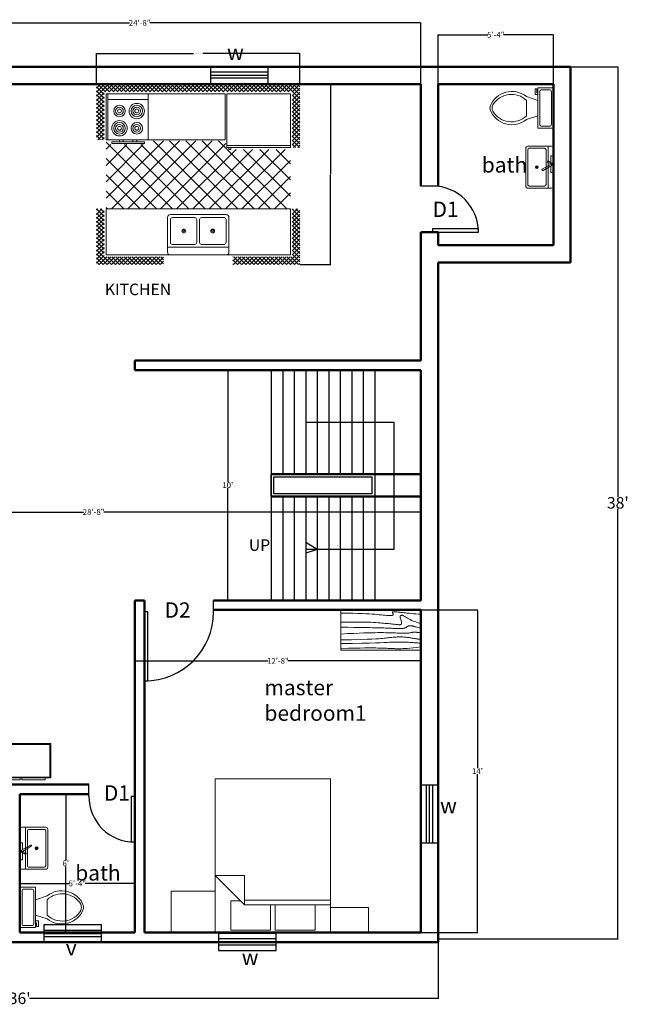
# Model space of a CAD drawing. Units: inches. Extents: x -10 to 557, y -66 to 886.
# Tile 3 of 6: x 241 to 557, y -65 to 448. Entities that reach past the tile are written whole.
import ezdxf

# ---------------------------------------------------------------- set-up
doc = ezdxf.new("R2010")
doc.units = ezdxf.units.IN
doc.header["$MEASUREMENT"] = 0
for name, color, linetype, lineweight in [('A-ANNO-DIMS', 2, 'Continuous', 18), ('A-ANNO-TEXT', 7, 'Continuous', 18), ('A-AREA-IDEN', 7, 'Continuous', 25), ('A-DOOR', 4, 'Continuous', 25), ('A-FLOR-FIXT', 8, 'Continuous', 18), ('A-FLOR-STRS', 3, 'Continuous', 25), ('A-FURN', 8, 'Continuous', 18), ('A-GLAZ', 4, 'Continuous', 25), ('A-WALL', 7, 'Continuous', 50)]:
    doc.layers.add(name, color=color, linetype=linetype, lineweight=lineweight)
doc.styles.get("Standard").update_dxf_attribs({"font": 'arial.ttf'})
doc.dimstyles.get("Standard").update_dxf_attribs({"dimtxt": 0.3, "dimasz": 0.4, "dimexe": 0.18, "dimexo": 0.0625, "dimgap": 0.09, "dimtad": 0, "dimtih": 1, "dimtoh": 1, "dimdec": 0, "dimrnd": 8, "dimzin": 0, "dimdsep": 46, "dimlunit": 3, "dimtxsty": 'Standard', "dimcen": 0.09, "dimadec": 0, "dimazin": 0, "dimtfac": 1, "dimtdec": 0, "dimtofl": 0, "dimtmove": 0, "dimatfit": 3, "dimfxl": 1, "dimtolj": 1, "dimtzin": 0, "dimarcsym": 0})

# ---------------------------------------------------------------- blocks, each defined once
blk = doc.blocks.new('*U30')
for p, q in [((0, 0), (0, 6)), ((24, 0), (24, 6))]:
    blk.add_line(p, q)
blk.add_lwpolyline([(0, 0), (0, -24), (1.75, -24), (1.75, 0)], close=True)
blk.add_arc((0, 0), 24, 270, 0)
blk = doc.blocks.new('*U29')
for p, q in [((0, 0), (0, 6)), ((36, 0), (36, 6))]:
    blk.add_line(p, q)
blk.add_lwpolyline([(0, 0), (0, -36), (1.75, -36), (1.75, 0)], close=True)
blk.add_arc((0, 0), 36, 270, 0)
blk = doc.blocks.new('*U31')
for p, q in [((0, 0), (0, -6)), ((24, 0), (24, -6))]:
    blk.add_line(p, q)
blk.add_lwpolyline([(0, 0), (0, 24), (1.75, 24), (1.75, 0)], close=True)
blk.add_arc((0, 0), 24, 0, 90)
blk = doc.blocks.new('Bed - Queen')
for p, q in [((0, -80.00003), (0, 0)), ((0, 0), (59.99999, 0)), ((59.99999, 0), (59.99999, -80.00003)), ((7.99999, -1.2), (28.79998, -1.2)), ((7.99999, -14.4), (7.99999, -1.2)), ((28.79998, -1.2), (28.79998, -14.4)), ((31.19999, -1.2), (51.99999, -1.2)), ((31.19999, -14.4), (31.19999, -1.2)), ((51.99999, -1.2), (51.99999, -16.4)), ((0, -14.4), (44.8, -14.4)), ((59.99999, -29.6), (44.8, -14.4)), ((44.8, -14.4), (44.8, -29.6)), ((44.8, -16.8), (0, -16.8)), ((51.99999, -16.4), (46.79936, -16.4)), ((44.8, -29.6), (59.99999, -29.6)), ((59.99999, -80.00003), (0, -80.00003))]:
    blk.add_line(p, q)
blk = doc.blocks.new('Toilet - top')
for p, q in [((9.5, -6), (9.5, -2)), ((-10, -8.5), (-8, -8.5)), ((-10, -9.5), (-10, -8.5)), ((-7, -9.5), (-10, -9.5)), ((-8, -8.5), (-8, -8)), ((-7, -8), (-7, -9.5)), ((-4, -8), (-6, -14)), ((4, -8), (6, -14)), ((4, -14), (-4, -14))]:
    blk.add_line(p, q)
blk.add_lwpolyline([(10.5, -8), (10.5, 0), (-10.5, 0), (-10.5, -8)], close=True)
for points in [[(-9.5, -2), (-9.5, -6)], [(8.5, -1), (-8.5, -1)], [(-8.5, -7), (8.5, -7)]]:
    blk.add_lwpolyline(points)
for centre, radius, start, end in [((-8.62, -1.88), 0.884, 81.8699, 188.1301), ((8.62, -1.88), 0.884, 351.8699, 98.1301), ((-8.62, -6.12), 0.884, 171.8699, 278.1301), ((8.62, -6.12), 0.884, 261.8699, 8.1301), ((3.52, -21.58), 12.17, 141.4691, 247.9714), ((4.2, -21.82), 11.33, 136.3677, 238.9468), ((-3.52, -21.58), 12.17, 292.0284, 38.5307), ((-4.2, -21.82), 11.33, 301.053, 43.6321), ((0, -27.88), 4, 245.7318, 294.2682), ((0, -29), 4, 254.8605, 285.1395)]:
    blk.add_arc(centre, radius, start, end)
blk = doc.blocks.new('Sink-single - 30 in top')
blk.add_line((-15, -3.999996), (15, -3.999996))
for points in [[(-13.5, 0), (13.5, 0)], [(-15, -18.499996), (-15, -1.5)], [(-13.5, -17.499996), (-13.5, -6.499996)], [(-12.5, -5.499996), (12.5, -5.499996)], [(13.5, -6.499996), (13.5, -17.499996)], [(15, -1.5), (15, -18.499996)], [(13.5, -19.999996), (-13.5, -19.999996)], [(12.5, -18.499996), (-12.5, -18.499996)]]:
    blk.add_lwpolyline(points)
for radius in [1, 0.5]:
    blk.add_circle((0, -11.999996), radius)
for centre, radius, start, end in [((-13.5, -1.5), 1.5, 90, 180), ((-12.5, -6.499996), 1, 90, 180), ((12.5, -6.499996), 1, 0, 90), ((13.5, -1.5), 1.5, 0, 90), ((-13.5, -18.499996), 1.5, 180, 270), ((-12.5, -17.499996), 1, 180, 270), ((12.5, -17.499996), 1, 270, 0), ((13.5, -18.499996), 1.5, 270, 0)]:
    blk.add_arc(centre, radius, start, end)
blk = doc.blocks.new('Faucet - single handle top')
for p, q in [((0.08, -0.26), (-2.26, -4.34)), ((-2.26, -4.34), (-1.37, -4.79)), ((-1.37, -4.79), (0.55, -0.5)), ((-0.06, -1.9), (3.57, -8.18)), ((4.43, -7.68), (0.72, -1.24))]:
    blk.add_line(p, q)
for points in [[(-0.92, -2), (-6, -2), (-6, 0), (6, 0), (6, -2), (1.16, -2)], [(-0.01, -2), (-0.12, -2)]]:
    blk.add_lwpolyline(points)
for centre, radius, start, end in [((0, -1), 0.75, 269.2246, 216.2304), ((4, -7.93), 0.5, 210, 30)]:
    blk.add_arc(centre, radius, start, end)
blk = doc.blocks.new('Table - Rectangular Woodgrain 60 x 30 in.')
for p, q in [((0, 0), (0, -30)), ((60, 0), (0, 0)), ((60, -30), (60, 0)), ((0, -30), (60, -30))]:
    blk.add_line(p, q)
for points in [[(0, -2.4), (4.8155, -2.418), (9.0302, -2.4688), (12.709, -2.5477), (15.9167, -2.65), (18.7181, -2.7711), (21.1781, -2.9063), (23.3616, -3.0508), (25.3333, -3.2), (27.1477, -3.3495), (28.8172, -3.4958), (30.3437, -3.636), (31.7291, -3.7667), (32.9756, -3.8849), (34.0849, -3.9875), (35.059, -4.0714), (35.9, -4.1334), (36.6114, -4.1711), (37.2041, -4.1854), (37.6906, -4.1779), (38.0833, -4.15), (38.3948, -4.1034), (38.6375, -4.0396), (38.8239, -3.9602), (38.9666, -3.8667), (39.0764, -3.7608), (39.1573, -3.6448), (39.2116, -3.521), (39.2416, -3.3917), (39.2498, -3.2593), (39.2385, -3.1261), (39.21, -2.9944), (39.1666, -2.8667), (39.111, -2.7447), (39.0468, -2.6281), (38.978, -2.5163), (38.9083, -2.4083), (38.8418, -2.3035), (38.7823, -2.201), (38.7337, -2.1001), (38.7, -2), (38.6844, -1.9003), (38.6875, -1.8021), (38.7094, -1.707), (38.75, -1.6167), (38.8094, -1.5326), (38.8875, -1.4563), (38.9844, -1.3893), (39.1, -1.3333), (39.2351, -1.2896), (39.3937, -1.2583), (39.5804, -1.2396), (39.8, -1.2333), (40.057, -1.2396), (40.3562, -1.2583), (40.7023, -1.2896), (41.1, -1.3333), (41.5547, -1.3895), (42.0755, -1.4573), (42.6721, -1.5361), (43.3542, -1.625), (44.1316, -1.7233), (45.014, -1.8302), (46.0114, -1.9449), (47.1333, -2.0667), (48.3862, -2.1947), (49.7625, -2.3281), (51.2513, -2.4663), (52.8416, -2.6083), (54.5226, -2.7535), (56.2833, -2.9011), (58.1127, -3.0501), (60, -3.2)], [(0, -9.2), (6.5759, -9.0858), (11.9385, -9.0365), (16.2527, -9.0418), (19.6833, -9.0917), (22.3952, -9.1759), (24.5531, -9.2844), (26.322, -9.4069), (27.8666, -9.5333), (29.3241, -9.6553), (30.7203, -9.7719), (32.0532, -9.8837), (33.3208, -9.9917), (34.5213, -10.0965), (35.6526, -10.199), (36.7128, -10.2999), (37.7, -10.4), (38.6129, -10.4996), (39.4531, -10.5969), (40.223, -10.6895), (40.925, -10.775), (41.5613, -10.8512), (42.1344, -10.9156), (42.6465, -10.966), (43.1, -11), (43.4976, -11.0158), (43.8437, -11.0136), (44.143, -10.9942), (44.4, -10.9583), (44.6195, -10.9069), (44.8062, -10.8406), (44.9648, -10.7603), (45.1, -10.6667), (45.2155, -10.5598), (45.3114, -10.4365), (45.3871, -10.2929), (45.4416, -10.125), (45.4743, -9.929), (45.4844, -9.7011), (45.4709, -9.4371), (45.4333, -9.1333), (45.3716, -8.7883), (45.2896, -8.4104), (45.1919, -8.0107), (45.0833, -7.6), (44.9685, -7.1893), (44.8521, -6.7896), (44.7388, -6.4117), (44.6333, -6.0667), (44.54, -5.7628), (44.4614, -5.4979), (44.4001, -5.2675), (44.3583, -5.0667), (44.3384, -4.8909), (44.3427, -4.7354), (44.3736, -4.5956), (44.4333, -4.4667), (44.5236, -4.3453), (44.6427, -4.2333), (44.7884, -4.1339), (44.9583, -4.05), (45.1501, -3.9849), (45.3614, -3.9417), (45.59, -3.9234), (45.8333, -3.9333), (46.0915, -3.9749), (46.3734, -4.0531), (46.6906, -4.1736), (47.0542, -4.3417), (47.4756, -4.5629), (47.9661, -4.8427), (48.5372, -5.1866), (49.2, -5.6), (49.9676, -6.0844), (50.8594, -6.625), (51.8965, -7.2031), (53.1, -7.8), (54.491, -8.3969), (56.0906, -8.975), (57.9199, -9.5156), (60, -10)], [(0, -12.8), (5.1847, -12.9322), (9.6213, -13.0323), (13.3963, -13.1059), (16.5958, -13.1583), (19.3063, -13.1952), (21.614, -13.2219), (23.6054, -13.2439), (25.3666, -13.2667), (26.9728, -13.2947), (28.4531, -13.3281), (29.8256, -13.3663), (31.1083, -13.4083), (32.3191, -13.4535), (33.476, -13.501), (34.597, -13.5501), (35.7, -13.6), (36.7984, -13.6497), (37.8875, -13.6979), (38.9578, -13.743), (40, -13.7833), (41.0047, -13.8174), (41.9625, -13.8438), (42.864, -13.8607), (43.7, -13.8667), (44.4631, -13.8604), (45.1552, -13.8417), (45.7801, -13.8104), (46.3416, -13.7667), (46.8439, -13.7104), (47.2906, -13.6417), (47.6858, -13.5604), (48.0333, -13.4667), (48.3375, -13.3608), (48.6042, -13.2448), (48.8396, -13.121), (49.05, -12.9917), (49.2417, -12.8593), (49.4208, -12.7261), (49.5937, -12.5944), (49.7667, -12.4667), (49.9452, -12.3451), (50.1323, -12.2313), (50.3303, -12.1268), (50.5416, -12.0333), (50.7686, -11.9524), (51.0135, -11.8854), (51.2788, -11.8341), (51.5666, -11.8), (51.8785, -11.7843), (52.2116, -11.7865), (52.562, -11.8059), (52.926, -11.8417), (53.2998, -11.8931), (53.6795, -11.9594), (54.0614, -12.0397), (54.4416, -12.1333), (54.8223, -12.2401), (55.2293, -12.3625), (55.6942, -12.5037), (56.2489, -12.6667), (56.9251, -12.8547), (57.7545, -13.0708), (58.7689, -13.3182), (60, -13.6)], [(0, -18), (5.124, -17.7273), (9.6609, -17.5057), (13.6705, -17.3303), (17.2125, -17.1958), (20.3467, -17.0973), (23.1328, -17.0297), (25.6307, -16.9878), (27.9, -16.9667), (29.9928, -16.9617), (31.9302, -16.9703), (33.7254, -16.9907), (35.3917, -17.0208), (36.9423, -17.0588), (38.3906, -17.1026), (39.7499, -17.1503), (41.0333, -17.2), (42.2519, -17.2496), (43.4073, -17.2969), (44.4986, -17.3395), (45.525, -17.375), (46.4858, -17.4012), (47.3802, -17.4156), (48.2074, -17.416), (48.9667, -17.4), (49.6583, -17.3662), (50.2872, -17.3167), (50.8595, -17.2547), (51.3812, -17.1833), (51.8584, -17.1057), (52.2971, -17.025), (52.7034, -16.9443), (53.0833, -16.8667), (53.443, -16.7951), (53.789, -16.7313), (54.128, -16.6768), (54.4666, -16.6334), (54.8115, -16.6024), (55.1693, -16.5854), (55.5465, -16.5841), (55.95, -16.6), (56.3828, -16.6337), (56.8346, -16.6823), (57.2915, -16.7418), (57.7396, -16.8084), (58.165, -16.878), (58.5539, -16.9469), (58.8924, -17.0111), (59.1666, -17.0667), (59.3679, -17.1107), (59.5078, -17.1438), (59.6032, -17.1675), (59.6708, -17.1833), (59.7275, -17.193), (59.7901, -17.1979), (59.8753, -17.1998), (60, -17.2)], [(0, -22.4), (8.0098, -22.2501), (14.4094, -22.1011), (19.4168, -21.9535), (23.25, -21.8083), (26.1269, -21.6663), (28.2656, -21.5281), (29.884, -21.3947), (31.2, -21.2667), (32.3967, -21.1448), (33.5172, -21.0292), (34.5697, -20.9198), (35.5625, -20.8167), (36.5037, -20.7198), (37.4015, -20.6292), (38.2642, -20.5448), (39.1, -20.4667), (39.9164, -20.3951), (40.7187, -20.3313), (41.5117, -20.2768), (42.3, -20.2333), (43.0883, -20.2024), (43.8812, -20.1854), (44.6836, -20.1841), (45.5, -20.2), (46.3328, -20.234), (47.1747, -20.2844), (48.0163, -20.3488), (48.8479, -20.425), (49.66, -20.5106), (50.4429, -20.6031), (51.1872, -20.7004), (51.8833, -20.8), (52.5246, -20.8999), (53.1166, -20.9995), (53.6681, -21.0983), (54.1875, -21.1958), (54.6834, -21.2919), (55.1646, -21.3859), (55.6394, -21.4777), (56.1167, -21.5667), (56.6028, -21.6515), (57.0961, -21.7266), (57.5929, -21.7852), (58.0896, -21.8208), (58.5823, -21.8268), (59.0674, -21.7964), (59.5412, -21.723), (60, -21.6)], [(0, -25.2), (8.6355, -25.0504), (15.7026, -24.9031), (21.4049, -24.7606), (25.9458, -24.625), (29.529, -24.4988), (32.3578, -24.3844), (34.6359, -24.284), (36.5667, -24.2), (38.3213, -24.1341), (39.9417, -24.0854), (41.437, -24.0523), (42.8167, -24.0333), (44.0901, -24.0268), (45.2667, -24.0313), (46.3557, -24.0451), (47.3667, -24.0667), (48.309, -24.0947), (49.1928, -24.1287), (50.0284, -24.168), (50.826, -24.2125), (51.5959, -24.2617), (52.3483, -24.3151), (53.0935, -24.3725), (53.8417, -24.4334), (54.6009, -24.497), (55.3699, -24.561), (56.1454, -24.6226), (56.9239, -24.6792), (57.7021, -24.7279), (58.4764, -24.7662), (59.2435, -24.7911), (60, -24.8)], [(0, -28.8), (5.6867, -28.6681), (10.45, -28.5698), (14.407, -28.5012), (17.675, -28.4584), (20.3711, -28.4374), (22.6125, -28.4344), (24.5164, -28.4455), (26.2, -28.4667), (27.762, -28.4947), (29.2276, -28.5281), (30.6033, -28.5663), (31.8958, -28.6084), (33.1118, -28.6535), (34.2578, -28.7011), (35.3405, -28.7501), (36.3666, -28.8), (37.3443, -28.8497), (38.288, -28.8974), (39.2137, -28.9412), (40.1375, -28.9792), (41.0753, -29.0093), (42.0432, -29.0297), (43.0572, -29.0384), (44.1333, -29.0333), (45.2936, -29.0114), (46.5843, -28.9641), (48.0579, -28.8816), (49.7666, -28.7542), (51.7629, -28.5721), (54.0989, -28.3255), (56.8272, -28.0048), (60, -27.6)]]:
    blk.add_lwpolyline(points)
blk = doc.blocks.new('Kitchen Layout - 7 x 8 ft')
for p, q in [((-5, 81.32), (2.68, 89)), ((-5, 83.44), (0.56, 89)), ((-5, 85.56), (-1.56, 89)), ((-5, 87.68), (-3.68, 89)), ((-1, 84.97), (-5, 88.97)), ((1.09, 85), (-2.91, 89)), ((3.21, 85), (-0.79, 89)), ((0.81, 85), (4.81, 89)), ((5.34, 85), (1.34, 89)), ((2.93, 85), (6.93, 89)), ((7.46, 85), (3.46, 89)), ((5.05, 85), (9.05, 89)), ((9.58, 85), (5.58, 89)), ((7.17, 85), (11.17, 89)), ((11.7, 85), (7.7, 89)), ((9.29, 85), (13.29, 89)), ((13.82, 85), (9.82, 89)), ((11.41, 85), (15.41, 89)), ((15.94, 85), (11.94, 89)), ((13.53, 85), (17.53, 89)), ((18.06, 85), (14.06, 89)), ((15.65, 85), (19.65, 89)), ((20.18, 85), (16.18, 89)), ((17.78, 85), (21.78, 89)), ((22.31, 85), (18.31, 89)), ((19.9, 85), (23.9, 89)), ((24.43, 85), (20.43, 89)), ((22.02, 85), (26.02, 89)), ((26.55, 85), (22.55, 89)), ((24.14, 85), (28.14, 89)), ((28.67, 85), (24.67, 89)), ((26.26, 85), (30.26, 89)), ((30.79, 85), (26.79, 89)), ((28.38, 85), (32.38, 89)), ((32.91, 85), (28.91, 89)), ((30.5, 85), (34.5, 89)), ((35.03, 85), (31.03, 89)), ((32.63, 85), (36.63, 89)), ((37.16, 85), (33.16, 89)), ((34.75, 85), (38.75, 89)), ((39.28, 85), (35.28, 89)), ((36.87, 85), (40.87, 89)), ((41.4, 85), (37.4, 89)), ((38.99, 85), (42.99, 89)), ((43.52, 85), (39.52, 89)), ((41.11, 85), (45.11, 89)), ((45.64, 85), (41.64, 89)), ((43.23, 85), (47.23, 89)), ((47.76, 85), (43.76, 89)), ((45.35, 85), (49.35, 89)), ((49.88, 85), (45.88, 89)), ((47.47, 85), (51.47, 89)), ((52, 85), (48, 89)), ((49.6, 85), (53.6, 89)), ((54.13, 85), (50.13, 89)), ((51.72, 85), (55.72, 89)), ((56.25, 85), (52.25, 89)), ((53.84, 85), (57.84, 89)), ((58.37, 85), (54.37, 89)), ((55.96, 85), (59.96, 89)), ((60.49, 85), (56.49, 89)), ((58.08, 85), (62.08, 89)), ((62.61, 85), (58.61, 89)), ((60.2, 85), (64.2, 89)), ((64.73, 85), (60.73, 89)), ((62.32, 85), (66.32, 89)), ((66.85, 85), (62.85, 89)), ((64.45, 85), (68.45, 89)), ((68.97, 85), (64.97, 89)), ((66.57, 85), (70.57, 89)), ((71.1, 85), (67.1, 89)), ((68.69, 85), (72.69, 89)), ((73.22, 85), (69.22, 89)), ((70.81, 85), (74.81, 89)), ((75.34, 85), (71.34, 89)), ((72.93, 85), (76.93, 89)), ((77.46, 85), (73.46, 89)), ((75.05, 85), (79.05, 89)), ((79.58, 85), (75.58, 89)), ((77.17, 85), (81.17, 89)), ((81.7, 85), (77.7, 89)), ((79.29, 85), (83.29, 89)), ((83.82, 85), (79.82, 89)), ((81.42, 85), (85.42, 89)), ((85.95, 85), (81.95, 89)), ((83.54, 85), (87.54, 89)), ((88.07, 85), (84.07, 89)), ((85.66, 85), (89.66, 89)), ((90.19, 85), (86.19, 89)), ((87.78, 85), (91.78, 89)), ((92.31, 85), (88.31, 89)), ((89.9, 85), (93.9, 89)), ((94.43, 85), (90.43, 89)), ((92.02, 85), (96.02, 89)), ((96.55, 85), (92.55, 89)), ((94.14, 85), (98.14, 89)), ((101, 82.67), (94.67, 89)), ((96.27, 85), (100.27, 89)), ((101, 84.79), (96.79, 89)), ((97, 83.61), (101, 87.61)), ((101, 86.92), (98.92, 89)), ((-1, 82.85), (-5, 86.85)), ((-1, 80.73), (-5, 84.73)), ((-5, 79.19), (-1, 83.19)), ((-1, 78.61), (-5, 82.61)), ((34, 84), (96, 84)), ((34, 60), (34, 84)), ((96, 84), (96, 60)), ((97, 81.49), (101, 85.49)), ((101, 80.55), (97, 84.55)), ((97, 79.37), (101, 83.37)), ((101, 78.43), (97, 82.43)), ((-5, 77.07), (-1, 81.07)), ((-1, 76.49), (-5, 80.49)), ((-5, 74.95), (-1, 78.95)), ((-1, 74.36), (-5, 78.36)), ((74, 81), (95, 81)), ((97, 77.25), (101, 81.25)), ((101, 76.31), (97, 80.31)), ((97, 75.13), (101, 79.13)), ((101, 74.19), (97, 78.19)), ((97, 73.01), (101, 77.01)), ((-5, 72.83), (-1, 76.83)), ((-1, 72.24), (-5, 76.24)), ((-5, 70.71), (-1, 74.71)), ((-1, 70.12), (-5, 74.12)), ((-5, 68.59), (-1, 72.59)), ((-1, 68), (-5, 72)), ((101, 72.07), (97, 76.07)), ((97, 70.89), (101, 74.89)), ((101, 69.95), (97, 73.95)), ((97, 68.76), (101, 72.76)), ((101, 67.82), (97, 71.82)), ((-5, 66.47), (-1, 70.47)), ((-1, 65.88), (-5, 69.88)), ((-5, 64.35), (-1, 68.35)), ((-1, 63.76), (-5, 67.76)), ((97, 66.64), (101, 70.64)), ((101, 65.7), (97, 69.7)), ((97, 64.52), (101, 68.52)), ((101, 63.58), (97, 67.58)), ((-5, 62.22), (-1, 66.22)), ((-1, 61.64), (-5, 65.64)), ((-5, 60.1), (-1, 64.1)), ((-1, 59.52), (-5, 63.52)), ((-5, 57.98), (-1, 61.98)), ((97, 62.4), (101, 66.4)), ((101, 61.46), (97, 65.46)), ((97, 60.28), (101, 64.28)), ((100.34, 60), (97, 63.34)), ((98.84, 60), (101, 62.16)), ((-1, 57.39), (-5, 61.39)), ((-1.73, 56), (-5, 59.27)), ((-3.85, 56), (-5, 57.15)), ((-4.86, 56), (-1, 59.86)), ((-2.74, 56), (-1, 57.74)), ((0, 57), (33, 57)), ((10.4, 24), (45.9, 59.5)), ((18.88, 24), (54.38, 59.5)), ((27.37, 24), (62.87, 59.5)), ((33.03, 55.11), (37.41, 59.5)), ((67.71, 24), (33.68, 58.04)), ((96, 60), (34, 60)), ((35.85, 24), (71.35, 59.5)), ((76.2, 24), (40.7, 59.5)), ((44.34, 24), (77.84, 57.5)), ((84.68, 24), (49.18, 59.5)), ((52.82, 24), (86.32, 57.5)), ((93.17, 24), (57.67, 59.5)), ((61.31, 24), (96, 58.69)), ((96, 29.65), (66.15, 59.5)), ((96, 38.14), (76.64, 57.5)), ((80, 60), (80, 59)), ((82, 59), (82, 60)), ((96, 46.63), (85.13, 57.5)), ((87, 59), (87, 60)), ((89, 60), (89, 59)), ((96, 55.11), (93.57, 57.54)), ((98.22, 60), (97, 61.22)), ((100.96, 60), (101, 60.04)), ((0, 30.57), (24.43, 55)), ((0, 39.06), (15.94, 55)), ((0, 47.54), (7.46, 55)), ((1.91, 24), (32.91, 55)), ((33.77, 24), (2.77, 55)), ((42.26, 24), (11.26, 55)), ((50.74, 24), (19.74, 55)), ((59.23, 24), (28.23, 55)), ((31, 55), (31, 56)), ((32, 55), (31, 55)), ((32, 56), (32, 55)), ((25.29, 24), (0, 49.29)), ((69.79, 24), (96, 50.21)), ((78.28, 24), (96, 41.72)), ((16.8, 24), (0, 40.8)), ((8.32, 24), (0, 32.32)), ((86.76, 24), (96, 33.24)), ((-5, 21.92), (-2.92, 24)), ((-5, 19.8), (-1, 23.8)), ((-1, 19.21), (-5, 23.21)), ((-5, 17.68), (-1, 21.68)), ((-1, 17.09), (-5, 21.09)), ((-1, 21.33), (-3.67, 24)), ((-1, 23.45), (-1.55, 24)), ((0, 24), (96, 24)), ((0, 0), (0, 24)), ((95.25, 24), (96, 24.75)), ((96, 24), (96, 0)), ((97, 22.1), (98.9, 24)), ((97, 19.97), (101, 23.97)), ((101, 19.03), (97, 23.03)), ((97, 17.85), (101, 21.85)), ((101, 16.91), (97, 20.91)), ((101, 21.16), (98.16, 24)), ((101, 23.28), (100.28, 24)), ((-5, 15.55), (-1, 19.55)), ((-1, 14.97), (-5, 18.97)), ((-5, 13.43), (-1, 17.43)), ((-1, 12.85), (-5, 16.85)), ((47.25, 6.5), (47.25, 18.5)), ((48.75, 18.5), (48.75, 6.5)), ((97, 15.73), (101, 19.73)), ((101, 14.79), (97, 18.79)), ((97, 13.61), (101, 17.61)), ((101, 12.67), (97, 16.67)), ((97, 11.49), (101, 15.49)), ((-5, 11.31), (-1, 15.31)), ((-1, 10.73), (-5, 14.73)), ((-5, 9.19), (-1, 13.19)), ((-1, 8.6), (-5, 12.6)), ((-5, 7.07), (-1, 11.07)), ((-1, 6.48), (-5, 10.48)), ((101, 10.55), (97, 14.55)), ((97, 9.37), (101, 13.37)), ((101, 8.43), (97, 12.43)), ((97, 7.25), (101, 11.25)), ((101, 6.31), (97, 10.31)), ((-5, 4.95), (-1, 8.95)), ((-1, 4.36), (-5, 8.36)), ((-5, 2.83), (-1, 6.83)), ((-1, 2.24), (-5, 6.24)), ((97, 5.12), (101, 9.12)), ((101, 4.18), (97, 8.18)), ((97, 3), (101, 7)), ((101, 2.06), (97, 6.06)), ((-5, 0.71), (-1, 4.71)), ((-1, 0.12), (-5, 4.12)), ((-5, -1.42), (-1, 2.58)), ((2, -5), (-5, 2)), ((-5, -3.54), (-1, 0.46)), ((96, 0), (0, 0)), ((64, 4), (32, 4)), ((93.24, -5), (101, 2.76)), ((95.36, -5), (101, 0.64)), ((97, 0.88), (101, 4.88)), ((101, -0.06), (97, 3.94)), ((101, -2.18), (97, 1.82)), ((-0.12, -5), (-5, -0.12)), ((-2.25, -5), (-5, -2.25)), ((-4.37, -5), (-5, -4.37)), ((-4.34, -5), (-0.34, -1)), ((-2.22, -5), (1.78, -1)), ((-0.1, -5), (3.9, -1)), ((4.12, -5), (0.12, -1)), ((2.02, -5), (6.02, -1)), ((6.24, -5), (2.24, -1)), ((4.14, -5), (8.14, -1)), ((8.36, -5), (4.36, -1)), ((6.27, -5), (10.27, -1)), ((10.48, -5), (6.48, -1)), ((8.39, -5), (12.39, -1)), ((12.6, -5), (8.6, -1)), ((10.51, -5), (14.51, -1)), ((14.73, -5), (10.73, -1)), ((12.63, -5), (16.63, -1)), ((16.85, -5), (12.85, -1)), ((14.75, -5), (18.75, -1)), ((18.97, -5), (14.97, -1)), ((16.87, -5), (20.87, -1)), ((21.09, -5), (17.09, -1)), ((18.99, -5), (22.99, -1)), ((23.21, -5), (19.21, -1)), ((21.11, -5), (25.11, -1)), ((25.33, -5), (21.33, -1)), ((23.24, -5), (27.24, -1)), ((27.45, -5), (23.45, -1)), ((25.36, -5), (29.36, -1)), ((29.57, -5), (25.57, -1)), ((27.48, -5), (30, -2.48)), ((30, -3.3), (27.7, -1)), ((29.6, -5), (30, -4.6)), ((30, -1.18), (29.82, -1)), ((66, -2.54), (67.54, -1)), ((66, -4.66), (69.66, -1)), ((69.88, -5), (66, -1.12)), ((67.76, -5), (66, -3.24)), ((67.78, -5), (71.78, -1)), ((72, -5), (68, -1)), ((69.9, -5), (73.9, -1)), ((74.12, -5), (70.12, -1)), ((72.03, -5), (76.03, -1)), ((76.24, -5), (72.24, -1)), ((74.15, -5), (78.15, -1)), ((78.36, -5), (74.36, -1)), ((76.27, -5), (80.27, -1)), ((80.49, -5), (76.49, -1)), ((78.39, -5), (82.39, -1)), ((82.61, -5), (78.61, -1)), ((80.51, -5), (84.51, -1)), ((84.73, -5), (80.73, -1)), ((82.63, -5), (86.63, -1)), ((86.85, -5), (82.85, -1)), ((84.75, -5), (88.75, -1)), ((88.97, -5), (84.97, -1)), ((86.88, -5), (90.88, -1)), ((91.09, -5), (87.09, -1)), ((89, -5), (93, -1)), ((93.21, -5), (89.21, -1)), ((91.12, -5), (95.12, -1)), ((95.34, -5), (91.34, -1)), ((97.46, -5), (93.46, -1)), ((99.58, -5), (95.58, -1)), ((101, -4.3), (97, -0.3)), ((97.48, -5), (101, -1.48)), ((99.6, -5), (101, -3.6))]:
    blk.add_line(p, q)
for points in [[(0, 56), (0, 84), (33, 84), (33, 56)], [(74, 60), (74, 84), (95, 84), (95, 60)], [(76, 58), (76, 59), (93, 59), (93, 58)]]:
    blk.add_lwpolyline(points, close=True)
for points in [[(33.5, 21), (62.5, 21)], [(32, 1.5), (32, 19.5)], [(33.5, 6.5), (33.5, 18.5)], [(34.5, 19.5), (46.25, 19.5)], [(49.75, 19.5), (61.5, 19.5)], [(62.5, 18.5), (62.5, 6.5)], [(64, 19.5), (64, 1.5)], [(46.25, 5.5), (34.5, 5.5)], [(61.5, 5.5), (49.75, 5.5)], [(62.5, 0), (33.5, 0)]]:
    blk.add_lwpolyline(points)
for centre, radius in [((80, 75), 4), ((80, 75), 3), ((80, 75), 2), ((89, 75), 3), ((89, 75), 2), ((80, 75), 1), ((89, 75), 1), ((80, 66), 3), ((80, 66), 2), ((80, 66), 1), ((89, 66), 4), ((89, 66), 3), ((89, 66), 2), ((89, 66), 1), ((40.5, 12.5), 1), ((40.5, 12.5), 0.5), ((55.5, 12.5), 1), ((55.5, 12.5), 0.5)]:
    blk.add_circle(centre, radius)
for centre, radius, start, end in [((33.5, 19.5), 1.5, 90, 180), ((62.5, 19.5), 1.5, 0, 90), ((34.5, 18.5), 1, 90, 180), ((46.25, 18.5), 1, 0, 90), ((49.75, 18.5), 1, 90, 180), ((61.5, 18.5), 1, 0, 90), ((34.5, 6.5), 1, 180, 270), ((46.25, 6.5), 1, 270, 0), ((49.75, 6.5), 1, 180, 270), ((61.5, 6.5), 1, 270, 0), ((33.5, 1.5), 1.5, 180, 270), ((62.5, 1.5), 1.5, 270, 0)]:
    blk.add_arc(centre, radius, start, end)
blk = doc.blocks.new('*D40')
at = {"layer": 'A-ANNO-DIMS', "color": 0, "lineweight": -2, "ltscale": 2, "transparency": 16777216}
for p, q in [((156.97, 414.38), (156.97, 446.36)), ((449.97, 414.38), (449.97, 446.36)), ((157.37, 446.18), (298.2, 446.18)), ((449.57, 446.18), (308.74, 446.18))]:
    blk.add_line(p, q, dxfattribs=at)
at = {"layer": 'A-ANNO-DIMS', "color": 0, "ltscale": 2, "transparency": 16777216}
for points in [[(157.37, 446.25), (157.37, 446.11), (156.97, 446.18)], [(449.57, 446.25), (449.57, 446.11), (449.97, 446.18)]]:
    blk.add_solid(points, dxfattribs=at)
at = {"layer": 'Defpoints', "color": 0, "ltscale": 2, "transparency": 16777216}
for p in [(449.97, 446.18), (156.97, 414.32), (449.97, 414.32)]:
    blk.add_point(p, dxfattribs=at)
at = {"layer": 'A-ANNO-DIMS', "color": 0, "ltscale": 2, "transparency": 16777216, "insert": (303.47, 446.18), "char_height": 0.3, "attachment_point": 5}
blk.add_mtext('\\A1;{\\H10x;24\'-8"}', dxfattribs=at)
blk = doc.blocks.new('*D41')
at = {"layer": 'A-ANNO-DIMS', "color": 0, "lineweight": -2, "ltscale": 2, "transparency": 16777216}
for p, q in [((458.97, 414.38), (458.97, 440.18)), ((459.37, 440), (484.89, 440)), ((518.57, 440), (493.05, 440)), ((518.97, 414.38), (518.97, 440.18))]:
    blk.add_line(p, q, dxfattribs=at)
at = {"layer": 'A-ANNO-DIMS', "color": 0, "ltscale": 2, "transparency": 16777216}
for points in [[(459.37, 440.06), (459.37, 439.93), (458.97, 440)], [(518.57, 440.06), (518.57, 439.93), (518.97, 440)]]:
    blk.add_solid(points, dxfattribs=at)
at = {"layer": 'Defpoints', "color": 0, "ltscale": 2, "transparency": 16777216}
for p in [(518.97, 440), (458.97, 414.32), (518.97, 414.32)]:
    blk.add_point(p, dxfattribs=at)
at = {"layer": 'A-ANNO-DIMS', "color": 0, "ltscale": 2, "transparency": 16777216, "insert": (488.97, 440), "char_height": 0.3, "attachment_point": 5}
blk.add_mtext('\\A1;{\\H10x;5\'-4"}', dxfattribs=at)
blk = doc.blocks.new('*D44')
at = {"layer": 'A-ANNO-DIMS', "color": 0, "lineweight": -2, "ltscale": 2, "transparency": 16777216}
for p, q in [((450.03, 140.32), (479.63, 140.32)), ((479.45, 139.92), (479.45, 57.92)), ((479.45, -27.28), (479.45, 54.73)), ((450.03, -27.68), (479.63, -27.68))]:
    blk.add_line(p, q, dxfattribs=at)
at = {"layer": 'A-ANNO-DIMS', "color": 0, "ltscale": 2, "transparency": 16777216}
for points in [[(479.39, 139.92), (479.52, 139.92), (479.45, 140.32)], [(479.39, -27.28), (479.52, -27.28), (479.45, -27.68)]]:
    blk.add_solid(points, dxfattribs=at)
at = {"layer": 'Defpoints', "color": 0, "ltscale": 2, "transparency": 16777216}
for p in [(449.97, 140.32), (449.97, -27.68), (479.45, -27.68)]:
    blk.add_point(p, dxfattribs=at)
at = {"layer": 'A-ANNO-DIMS', "color": 0, "ltscale": 2, "transparency": 16777216, "insert": (479.45, 56.32), "char_height": 0.3, "attachment_point": 5}
blk.add_mtext("\\A1;{\\H10x;14'}", dxfattribs=at)
blk = doc.blocks.new('*D45')
at = {"layer": 'A-ANNO-DIMS', "color": 0, "lineweight": -2, "ltscale": 2, "transparency": 16777216}
for p, q in [((300.97, 145.26), (300.97, 113.58)), ((449.97, 140.26), (449.97, 113.58)), ((301.37, 113.76), (370.37, 113.76)), ((449.57, 113.76), (380.57, 113.76))]:
    blk.add_line(p, q, dxfattribs=at)
at = {"layer": 'A-ANNO-DIMS', "color": 0, "ltscale": 2, "transparency": 16777216}
for points in [[(301.37, 113.82), (301.37, 113.69), (300.97, 113.76)], [(449.57, 113.82), (449.57, 113.69), (449.97, 113.76)]]:
    blk.add_solid(points, dxfattribs=at)
at = {"layer": 'Defpoints', "color": 0, "ltscale": 2, "transparency": 16777216}
for p in [(300.97, 145.32), (449.97, 140.32), (449.97, 113.76)]:
    blk.add_point(p, dxfattribs=at)
at = {"layer": 'A-ANNO-DIMS', "color": 0, "ltscale": 2, "transparency": 16777216, "insert": (375.47, 113.76), "char_height": 0.3, "attachment_point": 5}
blk.add_mtext('\\A1;{\\H10x;12\'-8"}', dxfattribs=at)
blk = doc.blocks.new('*D46')
at = {"layer": 'A-ANNO-DIMS', "color": 0, "lineweight": -2, "ltscale": 2, "transparency": 16777216}
for p, q in [((265, 43.92), (265, 9.94)), ((265.04, 44.32), (265.18, 44.32)), ((265, -27.28), (265, 6.7)), ((267.89, -27.68), (264.82, -27.68))]:
    blk.add_line(p, q, dxfattribs=at)
at = {"layer": 'A-ANNO-DIMS', "color": 0, "ltscale": 2, "transparency": 16777216}
for points in [[(264.94, 43.92), (265.07, 43.92), (265, 44.32)], [(264.94, -27.28), (265.07, -27.28), (265, -27.68)]]:
    blk.add_solid(points, dxfattribs=at)
at = {"layer": 'Defpoints', "color": 0, "ltscale": 2, "transparency": 16777216}
for p in [(264.98, 44.32), (265, -27.68), (267.95, -27.68)]:
    blk.add_point(p, dxfattribs=at)
at = {"layer": 'A-ANNO-DIMS', "color": 0, "ltscale": 2, "transparency": 16777216, "insert": (265, 8.32), "char_height": 0.3, "attachment_point": 5}
blk.add_mtext("\\A1;{\\H10x;6'}", dxfattribs=at)
blk = doc.blocks.new('*D47')
at = {"layer": 'A-ANNO-DIMS', "color": 0, "lineweight": -2, "ltscale": 2, "transparency": 16777216}
for p, q in [((240.97, -2.08), (240.97, -1.96)), ((241.37, -2.14), (266.89, -2.14)), ((300.57, -2.14), (275.05, -2.14)), ((300.97, -2.08), (300.97, -1.96))]:
    blk.add_line(p, q, dxfattribs=at)
at = {"layer": 'A-ANNO-DIMS', "color": 0, "ltscale": 2, "transparency": 16777216}
for points in [[(241.37, -2.07), (241.37, -2.21), (240.97, -2.14)], [(300.57, -2.07), (300.57, -2.21), (300.97, -2.14)]]:
    blk.add_solid(points, dxfattribs=at)
at = {"layer": 'Defpoints', "color": 0, "ltscale": 2, "transparency": 16777216}
for p in [(240.97, -2.14), (240.97, -2.14), (300.97, -2.14)]:
    blk.add_point(p, dxfattribs=at)
at = {"layer": 'A-ANNO-DIMS', "color": 0, "ltscale": 2, "transparency": 16777216, "insert": (270.97, -2.14), "char_height": 0.3, "attachment_point": 5}
blk.add_mtext('\\A1;{\\H10x;5\'-4"}', dxfattribs=at)
blk = doc.blocks.new('*D48')
at = {"layer": 'A-ANNO-DIMS', "color": 0, "lineweight": -2, "ltscale": 2, "transparency": 16777216}
for p, q in [((343.78, 265.32), (349.55, 265.32)), ((349.37, 264.92), (349.37, 206.94)), ((349.37, 145.72), (349.37, 203.7)), ((343.78, 145.32), (349.55, 145.32))]:
    blk.add_line(p, q, dxfattribs=at)
at = {"layer": 'A-ANNO-DIMS', "color": 0, "ltscale": 2, "transparency": 16777216}
for points in [[(349.31, 264.92), (349.44, 264.92), (349.37, 265.32)], [(349.31, 145.72), (349.44, 145.72), (349.37, 145.32)]]:
    blk.add_solid(points, dxfattribs=at)
at = {"layer": 'Defpoints', "color": 0, "ltscale": 2, "transparency": 16777216}
for p in [(343.72, 265.32), (343.72, 145.32), (349.37, 145.32)]:
    blk.add_point(p, dxfattribs=at)
at = {"layer": 'A-ANNO-DIMS', "color": 0, "ltscale": 2, "transparency": 16777216, "insert": (349.37, 205.32), "char_height": 0.3, "attachment_point": 5}
blk.add_mtext("\\A1;{\\H10x;10'}", dxfattribs=at)
blk = doc.blocks.new('*D49')
at = {"layer": 'A-ANNO-DIMS', "color": 0, "lineweight": -2, "ltscale": 2, "transparency": 16777216}
for p, q in [((108.97, 177.7), (108.97, 191.53)), ((109.37, 191.35), (274.2, 191.35)), ((449.57, 191.35), (284.74, 191.35)), ((449.97, 177.7), (449.97, 191.53))]:
    blk.add_line(p, q, dxfattribs=at)
at = {"layer": 'A-ANNO-DIMS', "color": 0, "ltscale": 2, "transparency": 16777216}
for points in [[(109.37, 191.42), (109.37, 191.28), (108.97, 191.35)], [(449.57, 191.42), (449.57, 191.28), (449.97, 191.35)]]:
    blk.add_solid(points, dxfattribs=at)
at = {"layer": 'Defpoints', "color": 0, "ltscale": 2, "transparency": 16777216}
for p in [(449.97, 191.35), (108.97, 177.64), (449.97, 177.64)]:
    blk.add_point(p, dxfattribs=at)
at = {"layer": 'A-ANNO-DIMS', "color": 0, "ltscale": 2, "transparency": 16777216, "insert": (279.47, 191.35), "char_height": 0.3, "attachment_point": 5}
blk.add_mtext('\\A1;{\\H10x;28\'-8"}', dxfattribs=at)
blk = doc.blocks.new('Entertainment Center')
for p, q in [((-4, 0), (-5, -1)), ((4, 0), (-4, 0)), ((5, -1), (4, 0)), ((-17, -19), (-17, -1)), ((-17, -1), (43, -1)), ((-16.5, -18.5), (-16.5, -1.5)), ((-16.5, -1.5), (42.5, -1.5)), ((42.5, -1.5), (42.5, -18.5)), ((43, -1), (43, -19)), ((43, -19), (-17, -19)), ((42.5, -18.5), (-16.5, -18.5)), ((-12, -20), (-12, -19)), ((12, -20), (-12, -20)), ((12, -19), (12, -20)), ((15, -20), (15, -19)), ((27, -20), (15, -20)), ((27, -19), (27, -20)), ((28, -20), (28, -19)), ((40, -20), (28, -20)), ((40, -19), (40, -20))]:
    blk.add_line(p, q)
blk.add_arc((0, 40), 61, 259.6111, 280.3889)
blk = doc.blocks.new('*D52')
at = {"layer": 'A-ANNO-DIMS', "color": 0, "lineweight": -2, "ltscale": 2, "transparency": 16777216}
for p, q in [((459.03, 423.32), (552.74, 423.32)), ((552.56, 422.92), (552.56, 199.28)), ((552.56, -30.68), (552.56, 192.97)), ((459.03, -31.08), (552.74, -31.08))]:
    blk.add_line(p, q, dxfattribs=at)
at = {"layer": 'A-ANNO-DIMS', "color": 0, "ltscale": 2, "transparency": 16777216}
for points in [[(552.49, 422.92), (552.63, 422.92), (552.56, 423.32)], [(552.49, -30.68), (552.63, -30.68), (552.56, -31.08)]]:
    blk.add_solid(points, dxfattribs=at)
at = {"layer": 'Defpoints', "color": 0, "ltscale": 2, "transparency": 16777216}
for p in [(458.97, 423.32), (458.97, -31.08), (552.56, -31.08)]:
    blk.add_point(p, dxfattribs=at)
at = {"layer": 'A-ANNO-DIMS', "color": 0, "ltscale": 2, "transparency": 16777216, "insert": (552.56, 196.12), "char_height": 0.3, "attachment_point": 5}
blk.add_mtext("\\A1;{\\H20x;38'}", dxfattribs=at)
blk = doc.blocks.new('*D53')
at = {"layer": 'A-ANNO-DIMS', "color": 0, "lineweight": -2, "ltscale": 2, "transparency": 16777216}
for p, q in [((22.97, -32.74), (22.97, -62.2)), ((458.97, -31.14), (458.97, -62.2)), ((23.37, -62.02), (235.79, -62.02)), ((458.57, -62.02), (246.15, -62.02))]:
    blk.add_line(p, q, dxfattribs=at)
at = {"layer": 'A-ANNO-DIMS', "color": 0, "ltscale": 2, "transparency": 16777216}
for points in [[(23.37, -61.96), (23.37, -62.09), (22.97, -62.02)], [(458.57, -61.96), (458.57, -62.09), (458.97, -62.02)]]:
    blk.add_solid(points, dxfattribs=at)
at = {"layer": 'Defpoints', "color": 0, "ltscale": 2, "transparency": 16777216}
for p in [(22.97, -32.68), (458.97, -31.08), (458.97, -62.02)]:
    blk.add_point(p, dxfattribs=at)
at = {"layer": 'A-ANNO-DIMS', "color": 0, "ltscale": 2, "transparency": 16777216, "insert": (240.97, -62.02), "char_height": 0.3, "attachment_point": 5}
blk.add_mtext("\\A1;{\\H20x;36'}", dxfattribs=at)
blk = doc.blocks.new('WIN-900')
for p, q in [((0, 6.25), (30, 6.25)), ((0, 4.5), (30, 4.5)), ((0, 3.05), (30, 3.05))]:
    blk.add_line(p, q)
blk.add_lwpolyline([(0, 9), (0, 0), (30, 0), (30, 9)], close=True)
blk = doc.blocks.new('*D77')
at = {"layer": 'A-ANNO-DIMS', "color": 0, "lineweight": -2, "ltscale": 2, "transparency": 16777216}
for p, q in [((280.95, 414.32), (280.95, 430.34)), ((281.35, 430.16), (331.47, 430.16)), ((386.55, 430.16), (336.42, 430.16)), ((386.95, 414.32), (386.95, 430.34))]:
    blk.add_line(p, q, dxfattribs=at)
at = {"layer": 'A-ANNO-DIMS', "color": 0, "ltscale": 2, "transparency": 16777216}
for points in [[(281.35, 430.22), (281.35, 430.09), (280.95, 430.16)], [(386.55, 430.22), (386.55, 430.09), (386.95, 430.16)]]:
    blk.add_solid(points, dxfattribs=at)
at = {"layer": 'Defpoints', "color": 0, "ltscale": 2, "transparency": 16777216}
for p in [(280.95, 430.16), (280.95, 414.26), (386.95, 414.26)]:
    blk.add_point(p, dxfattribs=at)
at = {"layer": 'A-ANNO-DIMS', "color": 0, "ltscale": 2, "transparency": 16777216, "insert": (333.95, 430.16), "char_height": 0.3, "attachment_point": 5}
blk.add_mtext('\\A1;KITCHEN LAYOUT 8\'-10"', dxfattribs=at)
blk = doc.blocks.new('*D78')
at = {"layer": 'A-ANNO-DIMS', "color": 0, "lineweight": -2, "ltscale": 2, "transparency": 16777216}
for p, q in [((387.01, 414.26), (403.03, 414.26)), ((402.85, 413.86), (402.85, 367.5)), ((402.85, 320.66), (402.85, 367.01)), ((387.01, 320.26), (403.03, 320.26))]:
    blk.add_line(p, q, dxfattribs=at)
at = {"layer": 'A-ANNO-DIMS', "color": 0, "ltscale": 2, "transparency": 16777216}
for points in [[(402.78, 413.86), (402.91, 413.86), (402.85, 414.26)], [(402.78, 320.66), (402.91, 320.66), (402.85, 320.26)]]:
    blk.add_solid(points, dxfattribs=at)
at = {"layer": 'Defpoints', "color": 0, "ltscale": 2, "transparency": 16777216}
for p in [(386.95, 414.26), (402.85, 414.26), (386.95, 320.26)]:
    blk.add_point(p, dxfattribs=at)
at = {"layer": 'A-ANNO-DIMS', "color": 0, "ltscale": 2, "transparency": 16777216, "insert": (402.85, 367.26), "char_height": 0.3, "attachment_point": 5}
blk.add_mtext('\\A1;7\'-10"', dxfattribs=at)

msp = doc.modelspace()

# ---------------------------------------------------------------- linework, layer by layer
at = {"layer": 'A-FLOR-STRS'}
for p, q in [((371.97, 265.32), (371.97, 145.32)), ((377.97, 265.32), (377.97, 211.15)), ((383.97, 265.32), (383.97, 211.15)), ((389.97, 265.32), (389.97, 211.15)), ((395.97, 265.32), (395.97, 211.15)), ((401.97, 265.32), (401.97, 211.15)), ((407.97, 265.32), (407.97, 211.15)), ((413.97, 265.32), (413.97, 211.15)), ((419.97, 265.32), (419.97, 211.15)), ((425.97, 265.32), (425.97, 145.32)), ((389.97, 238.24), (435.84, 238.24)), ((435.84, 238.24), (435.84, 171.74)), ((371.97, 199.49), (371.97, 211.15)), ((425.97, 211.15), (425.97, 199.49)), ((373.28, 209.66), (424.48, 209.66)), ((373.28, 200.85), (373.28, 209.66)), ((424.48, 209.66), (424.48, 200.85)), ((424.48, 200.85), (373.28, 200.85)), ((377.97, 199.49), (377.97, 145.32)), ((383.97, 199.49), (383.97, 145.32)), ((389.97, 199.49), (389.97, 145.32)), ((395.97, 199.49), (395.97, 145.32)), ((401.97, 199.49), (401.97, 145.32)), ((407.97, 199.49), (407.97, 145.32)), ((413.97, 199.49), (413.97, 145.32)), ((419.97, 199.49), (419.97, 145.32)), ((395.97, 171.74), (389.97, 175.52)), ((389.97, 175.52), (389.97, 169.89)), ((395.97, 174.52), (395.97, 168.29)), ((435.84, 171.74), (389.97, 171.74)), ((395.97, 171.74), (389.97, 169.89))]:
    msp.add_line(p, q, dxfattribs=at)
at = {"layer": 'A-FURN'}
for points in [[(342.88, -27.68), (342.88, -6.17), (319.93, -6.17), (319.93, -27.68)], [(402.88, -27.68), (402.88, -14.66), (422.59, -14.66), (422.59, -27.68)]]:
    msp.add_lwpolyline(points, close=True, dxfattribs=at)
at = {"layer": 'A-WALL'}
for p, q in [((22.97, 423.32), (382.97, 423.32)), ((382.97, 423.32), (458.97, 423.32)), ((458.97, 423.32), (527.97, 423.32)), ((527.97, 423.32), (527.97, 321.32)), ((156.97, 414.32), (449.97, 414.32)), ((449.97, 414.32), (449.97, 361.16)), ((458.97, 414.32), (458.97, 360.97)), ((458.97, 414.32), (518.97, 414.32)), ((458.97, 360.97), (458.97, 414.32)), ((518.97, 414.32), (518.97, 330.32)), ((449.97, 337.16), (458.97, 337.16)), ((449.97, 337.16), (449.97, 270.32)), ((458.97, 330.32), (458.97, 337.16)), ((458.97, 337.16), (458.97, 330.32)), ((518.97, 330.32), (458.97, 330.32)), ((527.97, 321.32), (458.97, 321.32)), ((458.97, 321.32), (458.97, -32.68)), ((300.97, 270.32), (449.97, 270.32)), ((300.97, 270.32), (300.97, 265.32)), ((300.97, 265.32), (449.97, 265.32)), ((449.97, 265.32), (449.97, 145.32)), ((371.97, 211.15), (449.97, 211.15)), ((449.97, 199.49), (371.97, 199.49)), ((300.97, 145.32), (300.97, 49.32)), ((305.97, 145.32), (300.97, 145.32)), ((305.97, 145.32), (305.97, 140.32)), ((341.97, 145.32), (449.97, 145.32)), ((305.97, 140.32), (305.97, -27.68)), ((341.97, 140.32), (449.97, 140.32)), ((449.97, 140.32), (449.97, -27.68)), ((108.97, 49.32), (276.97, 49.32)), ((300.97, 49.32), (300.97, 44.32)), ((240.97, 44.32), (240.97, -27.68)), ((240.97, 44.32), (276.97, 44.32)), ((300.97, 44.32), (300.97, -27.68)), ((240.97, -27.68), (300.97, -27.68)), ((305.97, -27.68), (449.97, -27.68)), ((22.97, -32.68), (458.97, -32.68))]:
    msp.add_line(p, q, dxfattribs=at)

# ---------------------------------------------------------------- block references
at = {"layer": 'A-DOOR'}
for name, p, rotation in [('*U30', (455.97, 337.16), 90), ('*U31', (300.97, 43.32), 180)]:
    msp.add_blockref(name, p, dxfattribs=dict(at, rotation=rotation))
msp.add_blockref('*U29', (305.97, 139.32), dxfattribs=at)
at = {"layer": 'A-FLOR-FIXT', "ltscale": 2, "xscale": -1}
msp.add_blockref('Kitchen Layout - 7 x 8 ft', (381.95, 325.26), dxfattribs=at)
at = {"layer": 'A-FLOR-FIXT'}
for p, rotation in [((518.93, 401.79), 270), ((241.25, -14.64), 89.99999999999999)]:
    msp.add_blockref('Toilet - top', p, dxfattribs=dict(at, rotation=rotation))
at = {"layer": 'A-FLOR-FIXT', "xscale": 0.7289455405337706, "yscale": 0.7289455405337706, "zscale": 0.7289455405337706}
for name, p, rotation in [('Sink-single - 30 in top', (519.15, 371), 270), ('Faucet - single handle top', (519.17, 372.58), 270), ('Sink-single - 30 in top', (241.03, 16.15), 89.99999999999999), ('Faucet - single handle top', (241, 14.57), 89.99999999999999)]:
    msp.add_blockref(name, p, dxfattribs=dict(at, rotation=rotation))
at = {"layer": 'A-FURN', "xscale": 0.6942880543039835, "yscale": 0.6942880543039835, "zscale": 0.6942880543039835}
msp.add_blockref('Table - Rectangular Woodgrain 60 x 30 in.', (408.3, 140.28), dxfattribs=at)
msp.add_blockref('Table - Rectangular Woodgrain 60 x 30 in.', (408.3, 140.28), dxfattribs=at)
msp.add_blockref('Table - Rectangular Woodgrain 60 x 30 in.', (408.3, 140.28), dxfattribs=at)
msp.add_blockref('Table - Rectangular Woodgrain 60 x 30 in.', (408.3, 140.28), dxfattribs=at)
at = {"layer": 'A-FURN'}
msp.add_blockref('Entertainment Center', (214.15, 71.78), dxfattribs=at)
at = {"layer": 'A-FURN', "rotation": 180}
msp.add_blockref('Bed - Queen', (402.88, -27.68), dxfattribs=at)
at = {"layer": 'A-GLAZ'}
for p in [(340.38, 414.48), (253.6, -32.77), (344.58, -37.18)]:
    msp.add_blockref('WIN-900', p, dxfattribs=at)
at = {"layer": 'A-GLAZ', "rotation": 270.0000000000003}
msp.add_blockref('WIN-900', (449.7, 49.05), dxfattribs=at)

# ---------------------------------------------------------------- texts
at = {"layer": 'A-ANNO-TEXT', "attachment_point": 1}
for s, width, insert, char_height in [('w', 13.506, (348.98, 434.79), 8), ('D1', 13.506, (456.04, 353.06), 8), ('UP', 11.6141, (360.35, 177.11), 6), ('D2', 13.506, (316.43, 144.26), 8), ('D1', 13.506, (284.83, 48.95), 8), ('w', 13.506, (459.95, 42.37), 8), ('v', 13.506, (264.99, -31.62), 8), ('w', 13.506, (356.61, -36.59), 8)]:
    msp.add_mtext_dynamic_manual_height_columns(s, width=width, gutter_width=1, heights=[0], dxfattribs=dict(at, insert=insert, char_height=char_height))
at = {"layer": 'A-AREA-IDEN', "char_height": 8, "attachment_point": 1}
for s, insert in [('bath', (481.68, 376.22)), (' master bedroom1', (368.49, 103.91)), ('bath', (269.91, 7.35))]:
    msp.add_mtext_dynamic_manual_height_columns(s, width=38.1538, gutter_width=1, heights=[0], dxfattribs=dict(at, insert=insert))
at = {"layer": 'A-AREA-IDEN', "ltscale": 2, "insert": (285.33, 310.32), "char_height": 6, "attachment_point": 1}
msp.add_mtext_dynamic_manual_height_columns('KITCHEN', width=61.8949, gutter_width=1, heights=[0], dxfattribs=at)

# ---------------------------------------------------------------- dimensions: what is measured, and where the dimension line sits
at = {"layer": 'A-ANNO-DIMS', "ltscale": 2}
for base, p1, p2, text, picture, middle in [((449.97, 446.18), (156.97, 414.32), (449.97, 414.32), '{\\H10x;<>}', '*D40', (303.47, 446.18)), ((518.97, 440), (458.97, 414.32), (518.97, 414.32), '{\\H10x;<>}', '*D41', (488.97, 440)), ((449.97, 191.35), (108.97, 177.64), (449.97, 177.64), '{\\H10x;<>}', '*D49', (279.47, 191.35)), ((449.97, 113.76), (300.97, 145.32), (449.97, 140.32), '{\\H10x;<>}', '*D45', (375.47, 113.76)), ((240.97, -2.14), (300.97, -2.14), (240.97, -2.14), '{\\H10x;<>}', '*D47', (270.97, -2.14)), ((458.97, -62.02), (22.97, -32.68), (458.97, -31.08), '{\\H20x;<>}', '*D53', (240.97, -62.02))]:
    dim = msp.add_linear_dim(base=base, p1=p1, p2=p2, text=text, dimstyle='Standard', override={"dimclrd": 0, "dimclre": 0, "dimclrt": 0}, dxfattribs=at)
    dim.commit()
    dim.dimension.update_dxf_attribs({"geometry": picture, "text_midpoint": middle})
for base, p1, p2, angle, text, override, picture, middle in [((280.95, 430.16), (386.95, 414.26), (280.95, 414.26), 180, 'KITCHEN LAYOUT <>', {"dimdec": 1, "dimrnd": 0, "dimzin": 1, "dimlunit": 4, "dimfrac": 2}, '*D77', (333.95, 430.16)), ((552.56, -31.08), (458.97, 423.32), (458.97, -31.08), 90, '{\\H20x;<>}', {"dimclrd": 0, "dimclre": 0, "dimclrt": 0}, '*D52', (552.56, 196.12)), ((349.37, 145.32), (343.72, 265.32), (343.72, 145.32), 90, '{\\H10x;<>}', {"dimclrd": 0, "dimclre": 0, "dimclrt": 0}, '*D48', (349.37, 205.32)), ((479.45, -27.68), (449.97, 140.32), (449.97, -27.68), 90, '{\\H10x;<>}', {"dimclrd": 0, "dimclre": 0, "dimclrt": 0}, '*D44', (479.45, 56.32)), ((265, -27.68), (264.98, 44.32), (267.95, -27.68), 90, '{\\H10x;<>}', {"dimclrd": 0, "dimclre": 0, "dimclrt": 0}, '*D46', (265, 8.32))]:
    dim = msp.add_linear_dim(base=base, p1=p1, p2=p2, angle=angle, text=text, dimstyle='Standard', override=override, dxfattribs=at)
    dim.commit()
    dim.dimension.update_dxf_attribs({"geometry": picture, "text_midpoint": middle})
dim = msp.add_linear_dim(base=(402.85, 414.26), p1=(386.95, 320.26), p2=(386.95, 414.26), angle=90, dimstyle='Standard', override={"dimdec": 1, "dimrnd": 0, "dimzin": 1, "dimlunit": 4, "dimfrac": 2}, dxfattribs=at)
dim.commit()
dim.dimension.update_dxf_attribs({"geometry": '*D78', "text_midpoint": (402.85, 367.26)})

doc.saveas('drawing.dxf')
